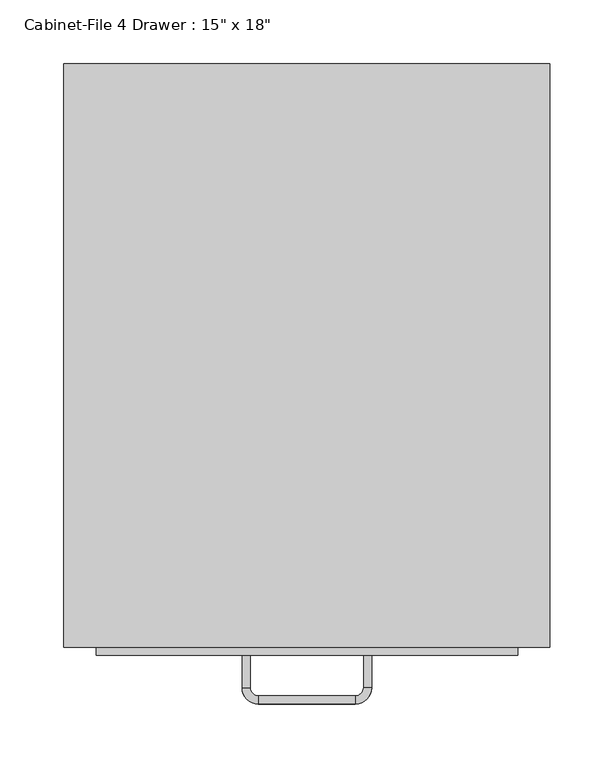
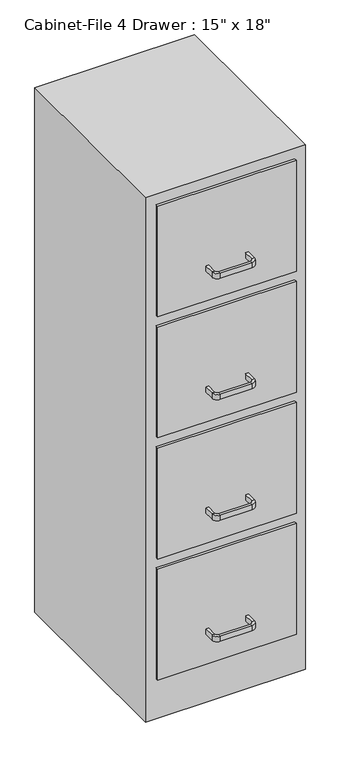
"""IFC4 building model written with IfcOpenShell, lengths in millimetres: furniture geometry."""

from ifc_helpers import new_model, si_unit, frame, origin, origin_with_axes, place, context, project, spatial, polyline, circle_curve, outline, extrude, source, transform, mapped, element, save
from ifc_brep_helpers import plane_surface, cylinder_surface, revolved_surface, advanced_brep


def furniture_b1353b55(model_context):
    return source(origin(), model_context, "Body", "SolidModel", [
        extrude(outline(polyline([(62.603553, 86.4656999), (62.603553, -370.7343001), (-318.396447, -370.7343001), (-318.396447, 86.4656999), (62.603553, 86.4656999)])), origin_with_axes(), (0.0, 0.0, 1.0), 1320.8),
        extrude(outline(polyline([(37.203553, -377.0843001), (-292.996447, -377.0843001), (-292.996447, -370.7343001), (37.203553, -370.7343001), (37.203553, -377.0843001)])), frame((0.0, 0.0, 1016.0), z_axis=(0.0, 0.0, 1.0), x_axis=(1.0, 0.0, 0.0)), (0.0, 0.0, 1.0), 279.4),
        extrude(outline(polyline([(37.203553, -377.0843001), (-292.996447, -377.0843001), (-292.996447, -370.7343001), (37.203553, -370.7343001), (37.203553, -377.0843001)])), frame((0.0, 0.0, 711.2), z_axis=(0.0, 0.0, 1.0), x_axis=(1.0, 0.0, 0.0)), (0.0, 0.0, 1.0), 279.4),
        extrude(outline(polyline([(37.203553, -377.0843001), (-292.996447, -377.0843001), (-292.996447, -370.7343001), (37.203553, -370.7343001), (37.203553, -377.0843001)])), frame((0.0, 0.0, 406.4), z_axis=(0.0, 0.0, 1.0), x_axis=(1.0, 0.0, 0.0)), (0.0, 0.0, 1.0), 279.4),
        extrude(outline(polyline([(37.203553, -377.0843001), (-292.996447, -377.0843001), (-292.996447, -370.7343001), (37.203553, -370.7343001), (37.203553, -377.0843001)])), frame((0.0, 0.0, 101.6), z_axis=(0.0, 0.0, 1.0), x_axis=(1.0, 0.0, 0.0)), (0.0, 0.0, 1.0), 279.4),
        advanced_brep(
        [(-172.346447, -377.0843001, 177.8), (-178.696447, -377.0843001, 177.8), (-178.696447, -377.0843001, 190.5), (-172.346447, -377.0843001, 190.5), (-172.346447, -402.4843001, 177.8), (-178.696447, -402.4843001, 177.8), (-178.696447, -402.4843001, 190.5), (-172.346447, -402.4843001, 190.5), (-165.996447, -415.1843001, 177.8), (-165.996447, -408.8343001, 177.8), (-165.996447, -415.1843001, 190.5), (-165.996447, -408.8343001, 190.5), (-89.796447, -408.8343001, 177.8), (-89.796447, -415.1843001, 177.8), (-89.796447, -415.1843001, 190.5), (-89.796447, -408.8343001, 190.5), (-77.096447, -402.4843001, 177.8), (-83.446447, -402.4843001, 177.8), (-77.096447, -402.4843001, 190.5), (-83.446447, -402.4843001, 190.5), (-83.446447, -377.0843001, 177.8), (-83.446447, -377.0843001, 190.5), (-77.096447, -377.0843001, 190.5), (-77.096447, -377.0843001, 177.8)],
        [
            (0, 1),
            (1, 2),
            (2, 3),
            (3, 0),
            (0, 4),
            (4, 5),
            (5, 1),
            (5, 6),
            (6, 2),
            (6, 7),
            (7, 3),
            (7, 4),
            (8, 5, circle_curve(frame((-165.996447, -402.4843001, 177.8), z_axis=(0.0, 0.0, -1.0), x_axis=(-1.0, 0.0, 0.0)), 12.7)),
            (4, 9, circle_curve(frame((-165.996447, -402.4843001, 177.8), z_axis=(0.0, 0.0, 1.0), x_axis=(-1.0, 0.0, 0.0)), 6.35)),
            (9, 8),
            (10, 6, circle_curve(frame((-165.996447, -402.4843001, 190.5), z_axis=(0.0, 0.0, -1.0), x_axis=(-1.0, 0.0, 0.0)), 12.7)),
            (8, 10),
            (11, 7, circle_curve(frame((-165.996447, -402.4843001, 190.5), z_axis=(0.0, 0.0, -1.0), x_axis=(-1.0, 0.0, 0.0)), 6.35)),
            (10, 11),
            (11, 9),
            (9, 12),
            (12, 13),
            (13, 8),
            (13, 14),
            (14, 10),
            (14, 15),
            (15, 11),
            (15, 12),
            (16, 13, circle_curve(frame((-89.796447, -402.4843001, 177.8), z_axis=(0.0, 0.0, -1.0), x_axis=(0.0, -1.0, 0.0)), 12.7)),
            (12, 17, circle_curve(frame((-89.796447, -402.4843001, 177.8), z_axis=(0.0, 0.0, 1.0), x_axis=(0.0, -1.0, 0.0)), 6.35)),
            (17, 16),
            (18, 14, circle_curve(frame((-89.796447, -402.4843001, 190.5), z_axis=(0.0, 0.0, -1.0), x_axis=(0.0, -1.0, 0.0)), 12.7)),
            (16, 18),
            (19, 15, circle_curve(frame((-89.796447, -402.4843001, 190.5), z_axis=(0.0, 0.0, -1.0), x_axis=(0.0, -1.0, 0.0)), 6.35)),
            (18, 19),
            (19, 17),
            (20, 21),
            (21, 22),
            (22, 23),
            (23, 20),
            (17, 20),
            (23, 16),
            (22, 18),
            (21, 19),
        ],
        [
            plane_surface(frame((-1283.614694, -377.0843001, 0.0), z_axis=(0.0, 1.0, 0.0), x_axis=(0.0, 0.0, -1.0))),
            plane_surface(frame((-172.346447, -377.0843001, 177.8), z_axis=(0.0, 0.0, -1.0), x_axis=(0.0, -1.0, 0.0))),
            plane_surface(frame((-178.696447, -377.0843001, 177.8), z_axis=(-1.0, 0.0, 0.0), x_axis=(0.0, -1.0, 0.0))),
            plane_surface(frame((-178.696447, -377.0843001, 190.5), z_axis=(0.0, 0.0, 1.0), x_axis=(0.0, -1.0, 0.0))),
            plane_surface(frame((-172.346447, -377.0843001, 190.5), z_axis=(1.0, 0.0, 0.0), x_axis=(0.0, -1.0, 0.0))),
            plane_surface(frame((-165.996447, -402.4843001, 177.8), z_axis=(0.0, 0.0, -1.0), x_axis=(-1.0, 0.0, 0.0))),
            cylinder_surface(frame((-165.996447, -402.4843001, 0.0), z_axis=(0.0, 0.0, 1.0), x_axis=(-1.0, 0.0, 0.0)), 12.7),
            plane_surface(frame((-165.996447, -402.4843001, 190.5), z_axis=(0.0, 0.0, 1.0), x_axis=(-1.0, 0.0, 0.0))),
            revolved_surface(polyline([(-172.34644699999998, -402.4843001, 190.5), (-172.34644699999998, -402.4843001, 177.8)]), (-165.996447, -402.4843001, 0.0), (0.0, 0.0, 1.0)),
            plane_surface(frame((-165.996447, -408.8343001, 177.8), z_axis=(0.0, 0.0, -1.0), x_axis=(1.0, 0.0, 0.0))),
            plane_surface(frame((-165.996447, -415.1843001, 177.8), z_axis=(0.0, -1.0, 0.0), x_axis=(1.0, 0.0, 0.0))),
            plane_surface(frame((-165.996447, -415.1843001, 190.5), z_axis=(0.0, 0.0, 1.0), x_axis=(1.0, 0.0, 0.0))),
            plane_surface(frame((-165.996447, -408.8343001, 190.5), z_axis=(0.0, 1.0, 0.0), x_axis=(1.0, 0.0, 0.0))),
            plane_surface(frame((-89.796447, -402.4843001, 177.8), z_axis=(0.0, 0.0, -1.0), x_axis=(0.0, -1.0, 0.0))),
            cylinder_surface(frame((-89.796447, -402.4843001, 0.0), z_axis=(0.0, 0.0, 1.0), x_axis=(0.0, -1.0, 0.0)), 12.7),
            plane_surface(frame((-89.796447, -402.4843001, 190.5), z_axis=(0.0, 0.0, 1.0), x_axis=(0.0, -1.0, 0.0))),
            revolved_surface(polyline([(-89.796447, -408.8343001, 190.5), (-89.796447, -408.8343001, 177.8)]), (-89.796447, -402.4843001, 0.0), (0.0, 0.0, 1.0)),
            plane_surface(frame((-1182.014694, -377.0843001, 0.0), z_axis=(0.0, 1.0, 0.0), x_axis=(0.0, 0.0, 1.0))),
            plane_surface(frame((-83.446447, -402.4843001, 177.8), z_axis=(0.0, 0.0, -1.0), x_axis=(0.0, 1.0, 0.0))),
            plane_surface(frame((-77.096447, -402.4843001, 177.8), z_axis=(1.0, 0.0, 0.0), x_axis=(0.0, 1.0, 0.0))),
            plane_surface(frame((-77.096447, -402.4843001, 190.5), z_axis=(0.0, 0.0, 1.0), x_axis=(0.0, 1.0, 0.0))),
            plane_surface(frame((-83.446447, -402.4843001, 190.5), z_axis=(-1.0, 0.0, 0.0), x_axis=(0.0, 1.0, 0.0))),
        ],
        [
            (0, [[1, 2, 3, 4]]),
            (1, [[-1, 5, 6, 7]]),
            (2, [[-2, -7, 8, 9]]),
            (3, [[-3, -9, 10, 11]]),
            (4, [[-4, -11, 12, -5]]),
            (5, [[13, -6, 14, 15]]),
            (6, [[16, -8, -13, 17]]),
            (7, [[18, -10, -16, 19]]),
            (8, [[-14, -12, -18, 20]]),
            (9, [[-15, 21, 22, 23]]),
            (10, [[-17, -23, 24, 25]]),
            (11, [[-19, -25, 26, 27]]),
            (12, [[-20, -27, 28, -21]]),
            (13, [[29, -22, 30, 31]]),
            (14, [[32, -24, -29, 33]]),
            (15, [[34, -26, -32, 35]]),
            (16, [[-30, -28, -34, 36]]),
            (17, [[37, 38, 39, 40]]),
            (18, [[-31, 41, -40, 42]]),
            (19, [[-33, -42, -39, 43]]),
            (20, [[-35, -43, -38, 44]]),
            (21, [[-36, -44, -37, -41]]),
        ],
    ),
        advanced_brep(
        [(-172.346447, -377.0843001, 482.6), (-178.696447, -377.0843001, 482.6), (-178.696447, -377.0843001, 495.3), (-172.346447, -377.0843001, 495.3), (-172.346447, -402.4843001, 482.6), (-178.696447, -402.4843001, 482.6), (-178.696447, -402.4843001, 495.3), (-172.346447, -402.4843001, 495.3), (-165.996447, -415.1843001, 482.6), (-165.996447, -408.8343001, 482.6), (-165.996447, -415.1843001, 495.3), (-165.996447, -408.8343001, 495.3), (-89.796447, -408.8343001, 482.6), (-89.796447, -415.1843001, 482.6), (-89.796447, -415.1843001, 495.3), (-89.796447, -408.8343001, 495.3), (-77.096447, -402.4843001, 482.6), (-83.446447, -402.4843001, 482.6), (-77.096447, -402.4843001, 495.3), (-83.446447, -402.4843001, 495.3), (-83.446447, -377.0843001, 482.6), (-83.446447, -377.0843001, 495.3), (-77.096447, -377.0843001, 495.3), (-77.096447, -377.0843001, 482.6)],
        [
            (0, 1),
            (1, 2),
            (2, 3),
            (3, 0),
            (0, 4),
            (4, 5),
            (5, 1),
            (5, 6),
            (6, 2),
            (6, 7),
            (7, 3),
            (7, 4),
            (8, 5, circle_curve(frame((-165.996447, -402.4843001, 482.6), z_axis=(0.0, 0.0, -1.0), x_axis=(-1.0, 0.0, 0.0)), 12.7)),
            (4, 9, circle_curve(frame((-165.996447, -402.4843001, 482.6), z_axis=(0.0, 0.0, 1.0), x_axis=(-1.0, 0.0, 0.0)), 6.35)),
            (9, 8),
            (10, 6, circle_curve(frame((-165.996447, -402.4843001, 495.3), z_axis=(0.0, 0.0, -1.0), x_axis=(-1.0, 0.0, 0.0)), 12.7)),
            (8, 10),
            (11, 7, circle_curve(frame((-165.996447, -402.4843001, 495.3), z_axis=(0.0, 0.0, -1.0), x_axis=(-1.0, 0.0, 0.0)), 6.35)),
            (10, 11),
            (11, 9),
            (9, 12),
            (12, 13),
            (13, 8),
            (13, 14),
            (14, 10),
            (14, 15),
            (15, 11),
            (15, 12),
            (16, 13, circle_curve(frame((-89.796447, -402.4843001, 482.6), z_axis=(0.0, 0.0, -1.0), x_axis=(0.0, -1.0, 0.0)), 12.7)),
            (12, 17, circle_curve(frame((-89.796447, -402.4843001, 482.6), z_axis=(0.0, 0.0, 1.0), x_axis=(0.0, -1.0, 0.0)), 6.35)),
            (17, 16),
            (18, 14, circle_curve(frame((-89.796447, -402.4843001, 495.3), z_axis=(0.0, 0.0, -1.0), x_axis=(0.0, -1.0, 0.0)), 12.7)),
            (16, 18),
            (19, 15, circle_curve(frame((-89.796447, -402.4843001, 495.3), z_axis=(0.0, 0.0, -1.0), x_axis=(0.0, -1.0, 0.0)), 6.35)),
            (18, 19),
            (19, 17),
            (20, 21),
            (21, 22),
            (22, 23),
            (23, 20),
            (17, 20),
            (23, 16),
            (22, 18),
            (21, 19),
        ],
        [
            plane_surface(frame((-1283.614694, -377.0843001, 0.0), z_axis=(0.0, 1.0, 0.0), x_axis=(0.0, 0.0, -1.0))),
            plane_surface(frame((-172.346447, -377.0843001, 482.6), z_axis=(0.0, 0.0, -1.0), x_axis=(0.0, -1.0, 0.0))),
            plane_surface(frame((-178.696447, -377.0843001, 482.6), z_axis=(-1.0, 0.0, 0.0), x_axis=(0.0, -1.0, 0.0))),
            plane_surface(frame((-178.696447, -377.0843001, 495.3), z_axis=(0.0, 0.0, 1.0), x_axis=(0.0, -1.0, 0.0))),
            plane_surface(frame((-172.346447, -377.0843001, 495.3), z_axis=(1.0, 0.0, 0.0), x_axis=(0.0, -1.0, 0.0))),
            plane_surface(frame((-165.996447, -402.4843001, 482.6), z_axis=(0.0, 0.0, -1.0), x_axis=(-1.0, 0.0, 0.0))),
            cylinder_surface(frame((-165.996447, -402.4843001, 0.0), z_axis=(0.0, 0.0, 1.0), x_axis=(-1.0, 0.0, 0.0)), 12.7),
            plane_surface(frame((-165.996447, -402.4843001, 495.3), z_axis=(0.0, 0.0, 1.0), x_axis=(-1.0, 0.0, 0.0))),
            revolved_surface(polyline([(-172.34644699999998, -402.4843001, 495.3), (-172.34644699999998, -402.4843001, 482.6)]), (-165.996447, -402.4843001, 0.0), (0.0, 0.0, 1.0)),
            plane_surface(frame((-165.996447, -408.8343001, 482.6), z_axis=(0.0, 0.0, -1.0), x_axis=(1.0, 0.0, 0.0))),
            plane_surface(frame((-165.996447, -415.1843001, 482.6), z_axis=(0.0, -1.0, 0.0), x_axis=(1.0, 0.0, 0.0))),
            plane_surface(frame((-165.996447, -415.1843001, 495.3), z_axis=(0.0, 0.0, 1.0), x_axis=(1.0, 0.0, 0.0))),
            plane_surface(frame((-165.996447, -408.8343001, 495.3), z_axis=(0.0, 1.0, 0.0), x_axis=(1.0, 0.0, 0.0))),
            plane_surface(frame((-89.796447, -402.4843001, 482.6), z_axis=(0.0, 0.0, -1.0), x_axis=(0.0, -1.0, 0.0))),
            cylinder_surface(frame((-89.796447, -402.4843001, 0.0), z_axis=(0.0, 0.0, 1.0), x_axis=(0.0, -1.0, 0.0)), 12.7),
            plane_surface(frame((-89.796447, -402.4843001, 495.3), z_axis=(0.0, 0.0, 1.0), x_axis=(0.0, -1.0, 0.0))),
            revolved_surface(polyline([(-89.796447, -408.8343001, 495.3), (-89.796447, -408.8343001, 482.6)]), (-89.796447, -402.4843001, 0.0), (0.0, 0.0, 1.0)),
            plane_surface(frame((-1182.014694, -377.0843001, 0.0), z_axis=(0.0, 1.0, 0.0), x_axis=(0.0, 0.0, 1.0))),
            plane_surface(frame((-83.446447, -402.4843001, 482.6), z_axis=(0.0, 0.0, -1.0), x_axis=(0.0, 1.0, 0.0))),
            plane_surface(frame((-77.096447, -402.4843001, 482.6), z_axis=(1.0, 0.0, 0.0), x_axis=(0.0, 1.0, 0.0))),
            plane_surface(frame((-77.096447, -402.4843001, 495.3), z_axis=(0.0, 0.0, 1.0), x_axis=(0.0, 1.0, 0.0))),
            plane_surface(frame((-83.446447, -402.4843001, 495.3), z_axis=(-1.0, 0.0, 0.0), x_axis=(0.0, 1.0, 0.0))),
        ],
        [
            (0, [[1, 2, 3, 4]]),
            (1, [[-1, 5, 6, 7]]),
            (2, [[-2, -7, 8, 9]]),
            (3, [[-3, -9, 10, 11]]),
            (4, [[-4, -11, 12, -5]]),
            (5, [[13, -6, 14, 15]]),
            (6, [[16, -8, -13, 17]]),
            (7, [[18, -10, -16, 19]]),
            (8, [[-14, -12, -18, 20]]),
            (9, [[-15, 21, 22, 23]]),
            (10, [[-17, -23, 24, 25]]),
            (11, [[-19, -25, 26, 27]]),
            (12, [[-20, -27, 28, -21]]),
            (13, [[29, -22, 30, 31]]),
            (14, [[32, -24, -29, 33]]),
            (15, [[34, -26, -32, 35]]),
            (16, [[-30, -28, -34, 36]]),
            (17, [[37, 38, 39, 40]]),
            (18, [[-31, 41, -40, 42]]),
            (19, [[-33, -42, -39, 43]]),
            (20, [[-35, -43, -38, 44]]),
            (21, [[-36, -44, -37, -41]]),
        ],
    ),
        advanced_brep(
        [(-172.346447, -377.0843001, 787.4), (-178.696447, -377.0843001, 787.4), (-178.696447, -377.0843001, 800.1), (-172.346447, -377.0843001, 800.1), (-172.346447, -402.4843001, 787.4), (-178.696447, -402.4843001, 787.4), (-178.696447, -402.4843001, 800.1), (-172.346447, -402.4843001, 800.1), (-165.996447, -415.1843001, 787.4), (-165.996447, -408.8343001, 787.4), (-165.996447, -415.1843001, 800.1), (-165.996447, -408.8343001, 800.1), (-89.796447, -408.8343001, 787.4), (-89.796447, -415.1843001, 787.4), (-89.796447, -415.1843001, 800.1), (-89.796447, -408.8343001, 800.1), (-77.096447, -402.4843001, 787.4), (-83.446447, -402.4843001, 787.4), (-77.096447, -402.4843001, 800.1), (-83.446447, -402.4843001, 800.1), (-83.446447, -377.0843001, 787.4), (-83.446447, -377.0843001, 800.1), (-77.096447, -377.0843001, 800.1), (-77.096447, -377.0843001, 787.4)],
        [
            (0, 1),
            (1, 2),
            (2, 3),
            (3, 0),
            (0, 4),
            (4, 5),
            (5, 1),
            (5, 6),
            (6, 2),
            (6, 7),
            (7, 3),
            (7, 4),
            (8, 5, circle_curve(frame((-165.996447, -402.4843001, 787.4), z_axis=(0.0, 0.0, -1.0), x_axis=(-1.0, 0.0, 0.0)), 12.7)),
            (4, 9, circle_curve(frame((-165.996447, -402.4843001, 787.4), z_axis=(0.0, 0.0, 1.0), x_axis=(-1.0, 0.0, 0.0)), 6.35)),
            (9, 8),
            (10, 6, circle_curve(frame((-165.996447, -402.4843001, 800.1), z_axis=(0.0, 0.0, -1.0), x_axis=(-1.0, 0.0, 0.0)), 12.7)),
            (8, 10),
            (11, 7, circle_curve(frame((-165.996447, -402.4843001, 800.1), z_axis=(0.0, 0.0, -1.0), x_axis=(-1.0, 0.0, 0.0)), 6.35)),
            (10, 11),
            (11, 9),
            (9, 12),
            (12, 13),
            (13, 8),
            (13, 14),
            (14, 10),
            (14, 15),
            (15, 11),
            (15, 12),
            (16, 13, circle_curve(frame((-89.796447, -402.4843001, 787.4), z_axis=(0.0, 0.0, -1.0), x_axis=(0.0, -1.0, 0.0)), 12.7)),
            (12, 17, circle_curve(frame((-89.796447, -402.4843001, 787.4), z_axis=(0.0, 0.0, 1.0), x_axis=(0.0, -1.0, 0.0)), 6.35)),
            (17, 16),
            (18, 14, circle_curve(frame((-89.796447, -402.4843001, 800.1), z_axis=(0.0, 0.0, -1.0), x_axis=(0.0, -1.0, 0.0)), 12.7)),
            (16, 18),
            (19, 15, circle_curve(frame((-89.796447, -402.4843001, 800.1), z_axis=(0.0, 0.0, -1.0), x_axis=(0.0, -1.0, 0.0)), 6.35)),
            (18, 19),
            (19, 17),
            (20, 21),
            (21, 22),
            (22, 23),
            (23, 20),
            (17, 20),
            (23, 16),
            (22, 18),
            (21, 19),
        ],
        [
            plane_surface(frame((-1283.614694, -377.0843001, 0.0), z_axis=(0.0, 1.0, 0.0), x_axis=(0.0, 0.0, -1.0))),
            plane_surface(frame((-172.346447, -377.0843001, 787.4), z_axis=(0.0, 0.0, -1.0), x_axis=(0.0, -1.0, 0.0))),
            plane_surface(frame((-178.696447, -377.0843001, 787.4), z_axis=(-1.0, 0.0, 0.0), x_axis=(0.0, -1.0, 0.0))),
            plane_surface(frame((-178.696447, -377.0843001, 800.1), z_axis=(0.0, 0.0, 1.0), x_axis=(0.0, -1.0, 0.0))),
            plane_surface(frame((-172.346447, -377.0843001, 800.1), z_axis=(1.0, 0.0, 0.0), x_axis=(0.0, -1.0, 0.0))),
            plane_surface(frame((-165.996447, -402.4843001, 787.4), z_axis=(0.0, 0.0, -1.0), x_axis=(-1.0, 0.0, 0.0))),
            cylinder_surface(frame((-165.996447, -402.4843001, 0.0), z_axis=(0.0, 0.0, 1.0), x_axis=(-1.0, 0.0, 0.0)), 12.7),
            plane_surface(frame((-165.996447, -402.4843001, 800.1), z_axis=(0.0, 0.0, 1.0), x_axis=(-1.0, 0.0, 0.0))),
            revolved_surface(polyline([(-172.34644699999998, -402.4843001, 800.1), (-172.34644699999998, -402.4843001, 787.4)]), (-165.996447, -402.4843001, 0.0), (0.0, 0.0, 1.0)),
            plane_surface(frame((-165.996447, -408.8343001, 787.4), z_axis=(0.0, 0.0, -1.0), x_axis=(1.0, 0.0, 0.0))),
            plane_surface(frame((-165.996447, -415.1843001, 787.4), z_axis=(0.0, -1.0, 0.0), x_axis=(1.0, 0.0, 0.0))),
            plane_surface(frame((-165.996447, -415.1843001, 800.1), z_axis=(0.0, 0.0, 1.0), x_axis=(1.0, 0.0, 0.0))),
            plane_surface(frame((-165.996447, -408.8343001, 800.1), z_axis=(0.0, 1.0, 0.0), x_axis=(1.0, 0.0, 0.0))),
            plane_surface(frame((-89.796447, -402.4843001, 787.4), z_axis=(0.0, 0.0, -1.0), x_axis=(0.0, -1.0, 0.0))),
            cylinder_surface(frame((-89.796447, -402.4843001, 0.0), z_axis=(0.0, 0.0, 1.0), x_axis=(0.0, -1.0, 0.0)), 12.7),
            plane_surface(frame((-89.796447, -402.4843001, 800.1), z_axis=(0.0, 0.0, 1.0), x_axis=(0.0, -1.0, 0.0))),
            revolved_surface(polyline([(-89.796447, -408.8343001, 800.1), (-89.796447, -408.8343001, 787.4)]), (-89.796447, -402.4843001, 0.0), (0.0, 0.0, 1.0)),
            plane_surface(frame((-1182.014694, -377.0843001, 0.0), z_axis=(0.0, 1.0, 0.0), x_axis=(0.0, 0.0, 1.0))),
            plane_surface(frame((-83.446447, -402.4843001, 787.4), z_axis=(0.0, 0.0, -1.0), x_axis=(0.0, 1.0, 0.0))),
            plane_surface(frame((-77.096447, -402.4843001, 787.4), z_axis=(1.0, 0.0, 0.0), x_axis=(0.0, 1.0, 0.0))),
            plane_surface(frame((-77.096447, -402.4843001, 800.1), z_axis=(0.0, 0.0, 1.0), x_axis=(0.0, 1.0, 0.0))),
            plane_surface(frame((-83.446447, -402.4843001, 800.1), z_axis=(-1.0, 0.0, 0.0), x_axis=(0.0, 1.0, 0.0))),
        ],
        [
            (0, [[1, 2, 3, 4]]),
            (1, [[-1, 5, 6, 7]]),
            (2, [[-2, -7, 8, 9]]),
            (3, [[-3, -9, 10, 11]]),
            (4, [[-4, -11, 12, -5]]),
            (5, [[13, -6, 14, 15]]),
            (6, [[16, -8, -13, 17]]),
            (7, [[18, -10, -16, 19]]),
            (8, [[-14, -12, -18, 20]]),
            (9, [[-15, 21, 22, 23]]),
            (10, [[-17, -23, 24, 25]]),
            (11, [[-19, -25, 26, 27]]),
            (12, [[-20, -27, 28, -21]]),
            (13, [[29, -22, 30, 31]]),
            (14, [[32, -24, -29, 33]]),
            (15, [[34, -26, -32, 35]]),
            (16, [[-30, -28, -34, 36]]),
            (17, [[37, 38, 39, 40]]),
            (18, [[-31, 41, -40, 42]]),
            (19, [[-33, -42, -39, 43]]),
            (20, [[-35, -43, -38, 44]]),
            (21, [[-36, -44, -37, -41]]),
        ],
    ),
        advanced_brep(
        [(-172.346447, -377.0843001, 1092.2), (-178.696447, -377.0843001, 1092.2), (-178.696447, -377.0843001, 1104.9), (-172.346447, -377.0843001, 1104.9), (-172.346447, -402.4843001, 1092.2), (-178.696447, -402.4843001, 1092.2), (-178.696447, -402.4843001, 1104.9), (-172.346447, -402.4843001, 1104.9), (-165.996447, -415.1843001, 1092.2), (-165.996447, -408.8343001, 1092.2), (-165.996447, -415.1843001, 1104.9), (-165.996447, -408.8343001, 1104.9), (-89.796447, -408.8343001, 1092.2), (-89.796447, -415.1843001, 1092.2), (-89.796447, -415.1843001, 1104.9), (-89.796447, -408.8343001, 1104.9), (-77.096447, -402.4843001, 1092.2), (-83.446447, -402.4843001, 1092.2), (-77.096447, -402.4843001, 1104.9), (-83.446447, -402.4843001, 1104.9), (-83.446447, -377.0843001, 1092.2), (-83.446447, -377.0843001, 1104.9), (-77.096447, -377.0843001, 1104.9), (-77.096447, -377.0843001, 1092.2)],
        [
            (0, 1),
            (1, 2),
            (2, 3),
            (3, 0),
            (0, 4),
            (4, 5),
            (5, 1),
            (5, 6),
            (6, 2),
            (6, 7),
            (7, 3),
            (7, 4),
            (8, 5, circle_curve(frame((-165.996447, -402.4843001, 1092.2), z_axis=(0.0, 0.0, -1.0), x_axis=(-1.0, 0.0, 0.0)), 12.7)),
            (4, 9, circle_curve(frame((-165.996447, -402.4843001, 1092.2), z_axis=(0.0, 0.0, 1.0), x_axis=(-1.0, 0.0, 0.0)), 6.35)),
            (9, 8),
            (10, 6, circle_curve(frame((-165.996447, -402.4843001, 1104.9), z_axis=(0.0, 0.0, -1.0), x_axis=(-1.0, 0.0, 0.0)), 12.7)),
            (8, 10),
            (11, 7, circle_curve(frame((-165.996447, -402.4843001, 1104.9), z_axis=(0.0, 0.0, -1.0), x_axis=(-1.0, 0.0, 0.0)), 6.35)),
            (10, 11),
            (11, 9),
            (9, 12),
            (12, 13),
            (13, 8),
            (13, 14),
            (14, 10),
            (14, 15),
            (15, 11),
            (15, 12),
            (16, 13, circle_curve(frame((-89.796447, -402.4843001, 1092.2), z_axis=(0.0, 0.0, -1.0), x_axis=(0.0, -1.0, 0.0)), 12.7)),
            (12, 17, circle_curve(frame((-89.796447, -402.4843001, 1092.2), z_axis=(0.0, 0.0, 1.0), x_axis=(0.0, -1.0, 0.0)), 6.35)),
            (17, 16),
            (18, 14, circle_curve(frame((-89.796447, -402.4843001, 1104.9), z_axis=(0.0, 0.0, -1.0), x_axis=(0.0, -1.0, 0.0)), 12.7)),
            (16, 18),
            (19, 15, circle_curve(frame((-89.796447, -402.4843001, 1104.9), z_axis=(0.0, 0.0, -1.0), x_axis=(0.0, -1.0, 0.0)), 6.35)),
            (18, 19),
            (19, 17),
            (20, 21),
            (21, 22),
            (22, 23),
            (23, 20),
            (17, 20),
            (23, 16),
            (22, 18),
            (21, 19),
        ],
        [
            plane_surface(frame((-1283.614694, -377.0843001, 0.0), z_axis=(0.0, 1.0, 0.0), x_axis=(0.0, 0.0, -1.0))),
            plane_surface(frame((-172.346447, -377.0843001, 1092.2), z_axis=(0.0, 0.0, -1.0), x_axis=(0.0, -1.0, 0.0))),
            plane_surface(frame((-178.696447, -377.0843001, 1092.2), z_axis=(-1.0, 0.0, 0.0), x_axis=(0.0, -1.0, 0.0))),
            plane_surface(frame((-178.696447, -377.0843001, 1104.9), z_axis=(0.0, 0.0, 1.0), x_axis=(0.0, -1.0, 0.0))),
            plane_surface(frame((-172.346447, -377.0843001, 1104.9), z_axis=(1.0, 0.0, 0.0), x_axis=(0.0, -1.0, 0.0))),
            plane_surface(frame((-165.996447, -402.4843001, 1092.2), z_axis=(0.0, 0.0, -1.0), x_axis=(-1.0, 0.0, 0.0))),
            cylinder_surface(frame((-165.996447, -402.4843001, 0.0), z_axis=(0.0, 0.0, 1.0), x_axis=(-1.0, 0.0, 0.0)), 12.7),
            plane_surface(frame((-165.996447, -402.4843001, 1104.9), z_axis=(0.0, 0.0, 1.0), x_axis=(-1.0, 0.0, 0.0))),
            revolved_surface(polyline([(-172.34644699999998, -402.4843001, 1104.9), (-172.34644699999998, -402.4843001, 1092.2)]), (-165.996447, -402.4843001, 0.0), (0.0, 0.0, 1.0)),
            plane_surface(frame((-165.996447, -408.8343001, 1092.2), z_axis=(0.0, 0.0, -1.0), x_axis=(1.0, 0.0, 0.0))),
            plane_surface(frame((-165.996447, -415.1843001, 1092.2), z_axis=(0.0, -1.0, 0.0), x_axis=(1.0, 0.0, 0.0))),
            plane_surface(frame((-165.996447, -415.1843001, 1104.9), z_axis=(0.0, 0.0, 1.0), x_axis=(1.0, 0.0, 0.0))),
            plane_surface(frame((-165.996447, -408.8343001, 1104.9), z_axis=(0.0, 1.0, 0.0), x_axis=(1.0, 0.0, 0.0))),
            plane_surface(frame((-89.796447, -402.4843001, 1092.2), z_axis=(0.0, 0.0, -1.0), x_axis=(0.0, -1.0, 0.0))),
            cylinder_surface(frame((-89.796447, -402.4843001, 0.0), z_axis=(0.0, 0.0, 1.0), x_axis=(0.0, -1.0, 0.0)), 12.7),
            plane_surface(frame((-89.796447, -402.4843001, 1104.9), z_axis=(0.0, 0.0, 1.0), x_axis=(0.0, -1.0, 0.0))),
            revolved_surface(polyline([(-89.796447, -408.8343001, 1104.9), (-89.796447, -408.8343001, 1092.2)]), (-89.796447, -402.4843001, 0.0), (0.0, 0.0, 1.0)),
            plane_surface(frame((-1182.014694, -377.0843001, 0.0), z_axis=(0.0, 1.0, 0.0), x_axis=(0.0, 0.0, 1.0))),
            plane_surface(frame((-83.446447, -402.4843001, 1092.2), z_axis=(0.0, 0.0, -1.0), x_axis=(0.0, 1.0, 0.0))),
            plane_surface(frame((-77.096447, -402.4843001, 1092.2), z_axis=(1.0, 0.0, 0.0), x_axis=(0.0, 1.0, 0.0))),
            plane_surface(frame((-77.096447, -402.4843001, 1104.9), z_axis=(0.0, 0.0, 1.0), x_axis=(0.0, 1.0, 0.0))),
            plane_surface(frame((-83.446447, -402.4843001, 1104.9), z_axis=(-1.0, 0.0, 0.0), x_axis=(0.0, 1.0, 0.0))),
        ],
        [
            (0, [[1, 2, 3, 4]]),
            (1, [[-1, 5, 6, 7]]),
            (2, [[-2, -7, 8, 9]]),
            (3, [[-3, -9, 10, 11]]),
            (4, [[-4, -11, 12, -5]]),
            (5, [[13, -6, 14, 15]]),
            (6, [[16, -8, -13, 17]]),
            (7, [[18, -10, -16, 19]]),
            (8, [[-14, -12, -18, 20]]),
            (9, [[-15, 21, 22, 23]]),
            (10, [[-17, -23, 24, 25]]),
            (11, [[-19, -25, 26, 27]]),
            (12, [[-20, -27, 28, -21]]),
            (13, [[29, -22, 30, 31]]),
            (14, [[32, -24, -29, 33]]),
            (15, [[34, -26, -32, 35]]),
            (16, [[-30, -28, -34, 36]]),
            (17, [[37, 38, 39, 40]]),
            (18, [[-31, 41, -40, 42]]),
            (19, [[-33, -42, -39, 43]]),
            (20, [[-35, -43, -38, 44]]),
            (21, [[-36, -44, -37, -41]]),
        ],
    ),
    ])


if __name__ == "__main__":
    model = new_model("IFC4")
    model_context = context("Model", 3, world=origin())
    ifc_project = project(units=[si_unit("LENGTHUNIT", "METRE", prefix="MILLI")], contexts=[model_context])
    site = spatial("IfcSite", under=ifc_project)
    building = spatial("IfcBuilding", under=site)
    placement = place(None, origin())
    furniture_shape = furniture_b1353b55(model_context)
    element("IfcFurniture", 1, ObjectType="Cabinet-File 4 Drawer : 15\" x 18\"", at=placement, inside=building, context=model_context, shape_type="MappedRepresentation", body=[
        mapped(furniture_shape, transform((0.0, 0.0, 0.0), x_axis=(1.0, 0.0, 0.0), y_axis=(0.0, 1.0, 0.0), z_axis=(0.0, 0.0, 1.0))),
    ])
    save(model, "model.ifc")

# Revit data of these elements
# Type "Cabinet-File 4 Drawer : 15\" x 18\""
#   Assembly Code = "E2020200"
#   Depth = 1' - 6"
#   Height = 4' - 4"
#   Width = 1' - 3"
#   Cabinet Material = Steel, Paint Finish, Ivory, Glossy
#   Handle Material = Steel, Chrome Plated
#   Default Elevation = 0
# Element 1 (IfcFurniture, "Cabinet-File 4 Drawer : 15\" x 18\"")
#   Materials on its faces: "Steel, Chrome Plated", "Steel, Paint Finish, Ivory, Glossy"
# Materials
#   "Steel, Paint Finish, Ivory, Glossy": class "Metal", colour RGB 247 247 239, transparency 0, Description = "Steel, paint finish, ivory, glossy", Cost = 0
#   "Steel, Chrome Plated": class "Metal", colour RGB 17 17 17, transparency 0, Description = "Chromiuim plated steel", Cost = 0
